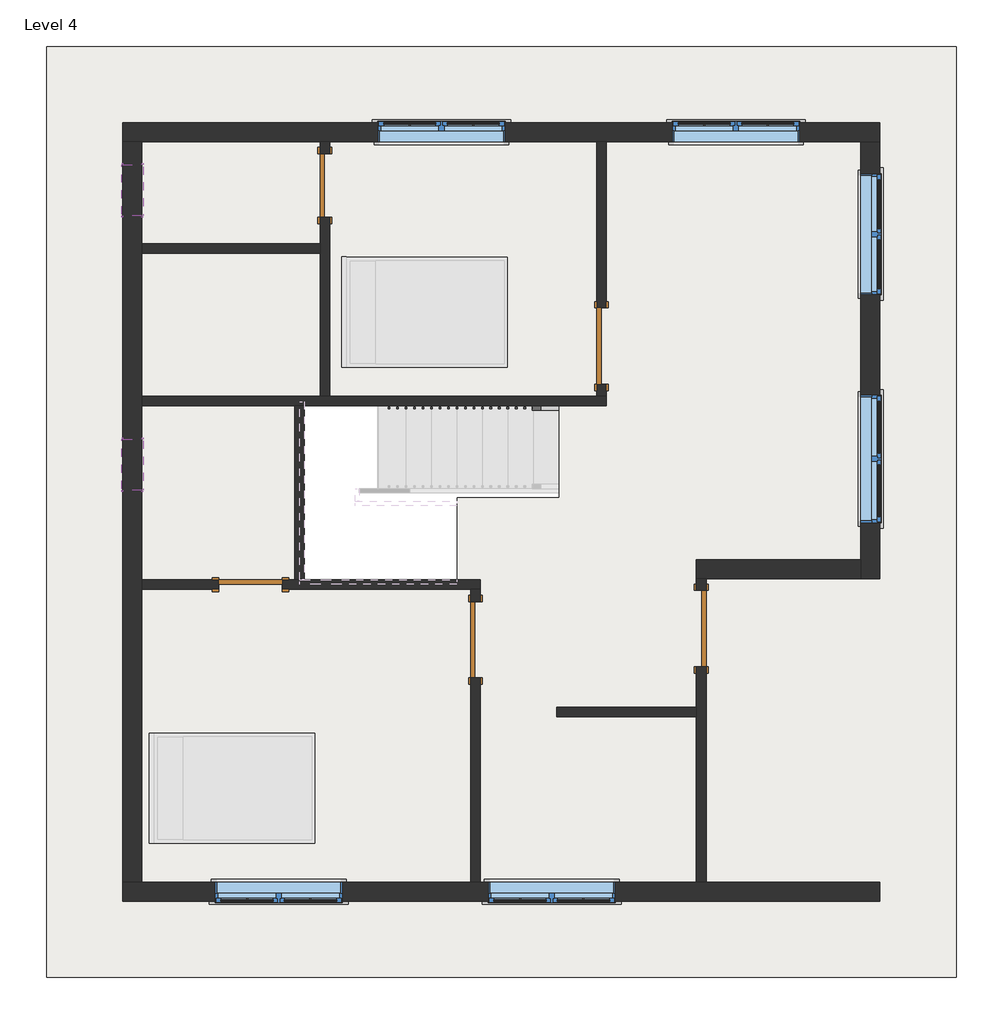
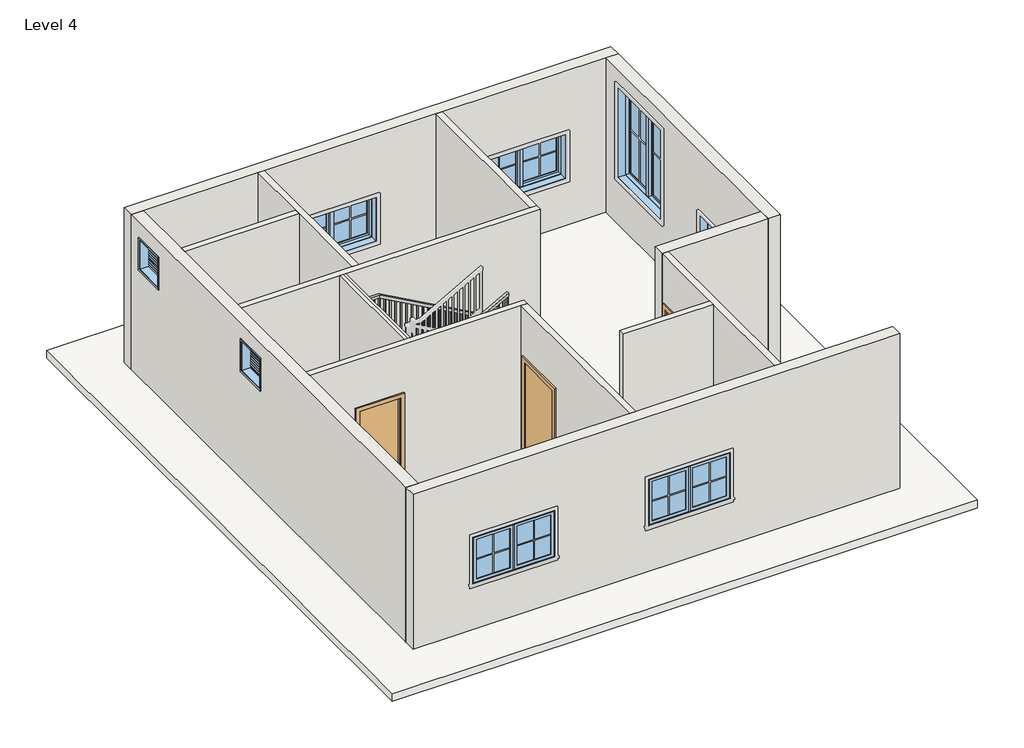
# One storey, part 1 of 2: 14 walls, 8 windows, 5 doors, 1 railing, 1 roof.
"""IFC4 building model written with IfcOpenShell, lengths in millimetres."""

from ifc_helpers import new_model, si_unit, frame, origin, place, context, project, spatial, polyline, outline, extrude, faceted_brep, transform, mapped, element, save
from components import single_flush_3_17d80c48, single_flush_3_5e62189b, door_d8f5dbb5, window_9ac97e1a, window_c1d95f0f, window_f2d8fef0

model = new_model("IFC4")

# Units and contexts
model_context = context("Model", 3, world=origin())
ifc_project = project(units=[si_unit("LENGTHUNIT", "METRE", prefix="MILLI")], contexts=[model_context])

# Site, building, storey
site = spatial("IfcSite", under=ifc_project)
building = spatial("IfcBuilding", under=site)
storey = spatial("IfcBuildingStorey", under=building, Name="Level 4", Elevation=9448.8)

# Doors
placement = place(None, origin())
single_flush_3_shape = single_flush_3_17d80c48(model_context)
element("IfcDoor", 1, ObjectType="Single-Flush : 3'", at=placement, inside=storey, context=model_context, shape_type="MappedRepresentation", body=[
    mapped(single_flush_3_shape, transform((-1566.5130704, -2143.0042021, 9448.8), x_axis=(0.0, 1.0, 0.0), y_axis=(-1.0, 0.0, 0.0), z_axis=(0.0, 0.0, 1.0))),
])
single_flush_3_2_shape = single_flush_3_5e62189b(model_context)
element("IfcDoor", 2, ObjectType="Single-Flush : 3'", at=placement, inside=storey, context=model_context, shape_type="MappedRepresentation", body=[
    mapped(single_flush_3_2_shape, transform((1138.5869296, -2009.6542021, 9448.8), x_axis=(0.0, 1.0, 0.0), y_axis=(-1.0, 0.0, 0.0), z_axis=(0.0, 0.0, 1.0))),
])
element("IfcDoor", 3, ObjectType="Single-Flush : 3'", at=placement, inside=storey, context=model_context, shape_type="MappedRepresentation", body=[
    mapped(single_flush_3_2_shape, transform((-55.2130704, 1374.8957979, 9448.8), x_axis=(0.0, -1.0, 0.0), y_axis=(1.0, 0.0, 0.0), z_axis=(0.0, 0.0, 1.0))),
])
door_shape = door_d8f5dbb5(model_context)
element("IfcDoor", 4, ObjectType="Single-Flush : DOOR 2'6\"", at=placement, inside=storey, context=model_context, shape_type="MappedRepresentation", body=[
    mapped(door_shape, transform((-3369.9130704, 3298.9457979, 9448.8), x_axis=(0.0, 1.0, 0.0), y_axis=(-1.0, 0.0, 0.0), z_axis=(0.0, 0.0, 1.0))),
])
element("IfcDoor", 5, ObjectType="Single-Flush : DOOR 2'6\"", at=placement, inside=storey, context=model_context, shape_type="MappedRepresentation", body=[
    mapped(door_shape, transform((-4258.9130704, -1482.6042021, 9448.8), x_axis=(1.0, 0.0, 0.0), y_axis=(0.0, 1.0, 0.0), z_axis=(0.0, 0.0, 1.0))),
])

# Railing
element("IfcRailing", 6, ObjectType="Handrail - Rectangular", at=placement, inside=storey, context=model_context, shape_type="SolidModel", body=[
    faceted_brep([(-569.5630704, 606.5457979, 10532.5333333), (-569.5630704, 606.5457979, 10474.420221), (-569.5630704, 657.3457979, 10474.420221), (-569.5630704, 657.3457979, 10532.5333333), (-3007.9630704, 606.5457979, 11887.2), (-3021.1266727, 606.5457979, 11836.4), (-3021.1266727, 657.3457979, 11836.4), (-3007.9630704, 657.3457979, 11887.2), (-3566.7630704, 606.5457979, 11887.2), (-3566.7630704, 606.5457979, 11836.4), (-3617.5630704, 657.3457979, 11836.4), (-3617.5630704, 657.3457979, 11887.2), (-3566.7630704, -1374.6542021, 11887.2), (-3566.7630704, -1374.6542021, 11836.4), (-3617.5630704, -1425.4542021, 11836.4), (-3617.5630704, -1425.4542021, 11887.2), (-3312.7630704, -1374.6542021, 11887.2), (-3299.5994682, -1374.6542021, 11836.4), (-3299.5994682, -1425.4542021, 11836.4), (-3312.7630704, -1425.4542021, 11887.2), (-1788.7630704, -1374.6542021, 12733.8666667), (-1788.7630704, -1425.4542021, 12733.8666667), (-1788.7630704, -1425.4542021, 12675.7535543), (-1788.7630704, -1374.6542021, 12675.7535543)], [[[0, 1, 2, 3]], [[1, 0, 4, 5]], [[2, 1, 5, 6]], [[3, 2, 6, 7]], [[0, 3, 7, 4]], [[5, 4, 8, 9]], [[6, 5, 9, 10]], [[7, 6, 10, 11]], [[4, 7, 11, 8]], [[9, 8, 12, 13]], [[10, 9, 13, 14]], [[11, 10, 14, 15]], [[8, 11, 15, 12]], [[13, 12, 16, 17]], [[14, 13, 17, 18]], [[15, 14, 18, 19]], [[12, 15, 19, 16]], [[20, 21, 22, 23]], [[17, 16, 20, 23]], [[18, 17, 23, 22]], [[19, 18, 22, 21]], [[16, 19, 21, 20]]]),
    extrude(outline(polyline([(12638.7118876, -1855.4380704), (12628.1285543, -1874.4880704), (11650.1333333, -1874.4880704), (11650.1333333, -1855.4380704), (12638.7118876, -1855.4380704)])), frame((0.0, -1409.5792021, 0.0), z_axis=(0.0, 1.0, 0.0), x_axis=(0.0, 0.0, 1.0)), (0.0, 0.0, 1.0), 19.05),
    extrude(outline(polyline([(12582.2674432, -1957.0380704), (12571.6841099, -1976.0880704), (11650.1333333, -1976.0880704), (11650.1333333, -1957.0380704), (12582.2674432, -1957.0380704)])), frame((0.0, -1409.5792021, 0.0), z_axis=(0.0, 1.0, 0.0), x_axis=(0.0, 0.0, 1.0)), (0.0, 0.0, 1.0), 19.05),
    extrude(outline(polyline([(12525.8229988, -2058.6380704), (12515.2396654, -2077.6880704), (11650.1333333, -2077.6880704), (11650.1333333, -2058.6380704), (12525.8229988, -2058.6380704)])), frame((0.0, -1409.5792021, 0.0), z_axis=(0.0, 1.0, 0.0), x_axis=(0.0, 0.0, 1.0)), (0.0, 0.0, 1.0), 19.05),
    extrude(outline(polyline([(12469.3785543, -2160.2380704), (12458.795221, -2179.2880704), (11480.8, -2179.2880704), (11480.8, -2160.2380704), (12469.3785543, -2160.2380704)])), frame((0.0, -1409.5792021, 0.0), z_axis=(0.0, 1.0, 0.0), x_axis=(0.0, 0.0, 1.0)), (0.0, 0.0, 1.0), 19.05),
    extrude(outline(polyline([(12412.9341099, -2261.8380704), (12402.3507765, -2280.8880704), (11480.8, -2280.8880704), (11480.8, -2261.8380704), (12412.9341099, -2261.8380704)])), frame((0.0, -1409.5792021, 0.0), z_axis=(0.0, 1.0, 0.0), x_axis=(0.0, 0.0, 1.0)), (0.0, 0.0, 1.0), 19.05),
    extrude(outline(polyline([(12356.4896654, -2363.4380704), (12345.9063321, -2382.4880704), (11480.8, -2382.4880704), (11480.8, -2363.4380704), (12356.4896654, -2363.4380704)])), frame((0.0, -1409.5792021, 0.0), z_axis=(0.0, 1.0, 0.0), x_axis=(0.0, 0.0, 1.0)), (0.0, 0.0, 1.0), 19.05),
    extrude(outline(polyline([(12300.045221, -2465.0380704), (12289.4618876, -2484.0880704), (11311.4666667, -2484.0880704), (11311.4666667, -2465.0380704), (12300.045221, -2465.0380704)])), frame((0.0, -1409.5792021, 0.0), z_axis=(0.0, 1.0, 0.0), x_axis=(0.0, 0.0, 1.0)), (0.0, 0.0, 1.0), 19.05),
    extrude(outline(polyline([(12243.6007765, -2566.6380704), (12233.0174432, -2585.6880704), (11311.4666667, -2585.6880704), (11311.4666667, -2566.6380704), (12243.6007765, -2566.6380704)])), frame((0.0, -1409.5792021, 0.0), z_axis=(0.0, 1.0, 0.0), x_axis=(0.0, 0.0, 1.0)), (0.0, 0.0, 1.0), 19.05),
    extrude(outline(polyline([(12187.1563321, -2668.2380704), (12176.5729988, -2687.2880704), (11311.4666667, -2687.2880704), (11311.4666667, -2668.2380704), (12187.1563321, -2668.2380704)])), frame((0.0, -1409.5792021, 0.0), z_axis=(0.0, 1.0, 0.0), x_axis=(0.0, 0.0, 1.0)), (0.0, 0.0, 1.0), 19.05),
    extrude(outline(polyline([(12130.7118876, -2769.8380704), (12120.1285543, -2788.8880704), (11142.1333333, -2788.8880704), (11142.1333333, -2769.8380704), (12130.7118876, -2769.8380704)])), frame((0.0, -1409.5792021, 0.0), z_axis=(0.0, 1.0, 0.0), x_axis=(0.0, 0.0, 1.0)), (0.0, 0.0, 1.0), 19.05),
    extrude(outline(polyline([(12074.2674432, -2871.4380704), (12063.6841099, -2890.4880704), (11142.1333333, -2890.4880704), (11142.1333333, -2871.4380704), (12074.2674432, -2871.4380704)])), frame((0.0, -1409.5792021, 0.0), z_axis=(0.0, 1.0, 0.0), x_axis=(0.0, 0.0, 1.0)), (0.0, 0.0, 1.0), 19.05),
    extrude(outline(polyline([(12017.8229988, -2973.0380704), (12007.2396654, -2992.0880704), (11142.1333333, -2992.0880704), (11142.1333333, -2973.0380704), (12017.8229988, -2973.0380704)])), frame((0.0, -1409.5792021, 0.0), z_axis=(0.0, 1.0, 0.0), x_axis=(0.0, 0.0, 1.0)), (0.0, 0.0, 1.0), 19.05),
    extrude(outline(polyline([(11961.3785543, -3074.6380704), (11950.795221, -3093.6880704), (10972.8, -3093.6880704), (10972.8, -3074.6380704), (11961.3785543, -3074.6380704)])), frame((0.0, -1409.5792021, 0.0), z_axis=(0.0, 1.0, 0.0), x_axis=(0.0, 0.0, 1.0)), (0.0, 0.0, 1.0), 19.05),
    extrude(outline(polyline([(11904.9341099, -3176.2380704), (11894.3507765, -3195.2880704), (10972.8, -3195.2880704), (10972.8, -3176.2380704), (11904.9341099, -3176.2380704)])), frame((0.0, -1409.5792021, 0.0), z_axis=(0.0, 1.0, 0.0), x_axis=(0.0, 0.0, 1.0)), (0.0, 0.0, 1.0), 19.05),
    extrude(outline(polyline([(11848.4896654, -3277.8380704), (11837.9063321, -3296.8880704), (10972.8, -3296.8880704), (10972.8, -3277.8380704), (11848.4896654, -3277.8380704)])), frame((0.0, -1409.5792021, 0.0), z_axis=(0.0, 1.0, 0.0), x_axis=(0.0, 0.0, 1.0)), (0.0, 0.0, 1.0), 19.05),
    extrude(outline(polyline([(-3398.4880704, -1409.5792021), (-3398.4880704, -1390.5292021), (-3379.4380704, -1390.5292021), (-3379.4380704, -1409.5792021), (-3398.4880704, -1409.5792021)])), frame((0.0, 0.0, 10972.8), z_axis=(0.0, 0.0, 1.0), x_axis=(1.0, 0.0, 0.0)), (0.0, 0.0, 1.0), 863.6),
    extrude(outline(polyline([(-3500.0880704, -1409.5792021), (-3500.0880704, -1390.5292021), (-3481.0380704, -1390.5292021), (-3481.0380704, -1409.5792021), (-3500.0880704, -1409.5792021)])), frame((0.0, 0.0, 10972.8), z_axis=(0.0, 0.0, 1.0), x_axis=(1.0, 0.0, 0.0)), (0.0, 0.0, 1.0), 863.6),
    extrude(outline(polyline([(-3601.6880704, -1288.9292021), (-3582.6380704, -1288.9292021), (-3582.6380704, -1307.9792021), (-3601.6880704, -1307.9792021), (-3601.6880704, -1288.9292021)])), frame((0.0, 0.0, 10972.8), z_axis=(0.0, 0.0, 1.0), x_axis=(1.0, 0.0, 0.0)), (0.0, 0.0, 1.0), 863.6),
    extrude(outline(polyline([(-3601.6880704, -1187.3292021), (-3582.6380704, -1187.3292021), (-3582.6380704, -1206.3792021), (-3601.6880704, -1206.3792021), (-3601.6880704, -1187.3292021)])), frame((0.0, 0.0, 10972.8), z_axis=(0.0, 0.0, 1.0), x_axis=(1.0, 0.0, 0.0)), (0.0, 0.0, 1.0), 863.6),
    extrude(outline(polyline([(-3601.6880704, -1085.7292021), (-3582.6380704, -1085.7292021), (-3582.6380704, -1104.7792021), (-3601.6880704, -1104.7792021), (-3601.6880704, -1085.7292021)])), frame((0.0, 0.0, 10972.8), z_axis=(0.0, 0.0, 1.0), x_axis=(1.0, 0.0, 0.0)), (0.0, 0.0, 1.0), 863.6),
    extrude(outline(polyline([(-3601.6880704, -984.1292021), (-3582.6380704, -984.1292021), (-3582.6380704, -1003.1792021), (-3601.6880704, -1003.1792021), (-3601.6880704, -984.1292021)])), frame((0.0, 0.0, 10972.8), z_axis=(0.0, 0.0, 1.0), x_axis=(1.0, 0.0, 0.0)), (0.0, 0.0, 1.0), 863.6),
    extrude(outline(polyline([(-3601.6880704, -882.5292021), (-3582.6380704, -882.5292021), (-3582.6380704, -901.5792021), (-3601.6880704, -901.5792021), (-3601.6880704, -882.5292021)])), frame((0.0, 0.0, 10972.8), z_axis=(0.0, 0.0, 1.0), x_axis=(1.0, 0.0, 0.0)), (0.0, 0.0, 1.0), 863.6),
    extrude(outline(polyline([(-3601.6880704, -780.9292021), (-3582.6380704, -780.9292021), (-3582.6380704, -799.9792021), (-3601.6880704, -799.9792021), (-3601.6880704, -780.9292021)])), frame((0.0, 0.0, 10972.8), z_axis=(0.0, 0.0, 1.0), x_axis=(1.0, 0.0, 0.0)), (0.0, 0.0, 1.0), 863.6),
    extrude(outline(polyline([(-3601.6880704, -679.3292021), (-3582.6380704, -679.3292021), (-3582.6380704, -698.3792021), (-3601.6880704, -698.3792021), (-3601.6880704, -679.3292021)])), frame((0.0, 0.0, 10972.8), z_axis=(0.0, 0.0, 1.0), x_axis=(1.0, 0.0, 0.0)), (0.0, 0.0, 1.0), 863.6),
    extrude(outline(polyline([(-3601.6880704, -577.7292021), (-3582.6380704, -577.7292021), (-3582.6380704, -596.7792021), (-3601.6880704, -596.7792021), (-3601.6880704, -577.7292021)])), frame((0.0, 0.0, 10972.8), z_axis=(0.0, 0.0, 1.0), x_axis=(1.0, 0.0, 0.0)), (0.0, 0.0, 1.0), 863.6),
    extrude(outline(polyline([(-3601.6880704, -476.1292021), (-3582.6380704, -476.1292021), (-3582.6380704, -495.1792021), (-3601.6880704, -495.1792021), (-3601.6880704, -476.1292021)])), frame((0.0, 0.0, 10972.8), z_axis=(0.0, 0.0, 1.0), x_axis=(1.0, 0.0, 0.0)), (0.0, 0.0, 1.0), 863.6),
    extrude(outline(polyline([(-3601.6880704, -374.5292021), (-3582.6380704, -374.5292021), (-3582.6380704, -393.5792021), (-3601.6880704, -393.5792021), (-3601.6880704, -374.5292021)])), frame((0.0, 0.0, 10972.8), z_axis=(0.0, 0.0, 1.0), x_axis=(1.0, 0.0, 0.0)), (0.0, 0.0, 1.0), 863.6),
    extrude(outline(polyline([(-3601.6880704, -272.9292021), (-3582.6380704, -272.9292021), (-3582.6380704, -291.9792021), (-3601.6880704, -291.9792021), (-3601.6880704, -272.9292021)])), frame((0.0, 0.0, 10972.8), z_axis=(0.0, 0.0, 1.0), x_axis=(1.0, 0.0, 0.0)), (0.0, 0.0, 1.0), 863.6),
    extrude(outline(polyline([(-3601.6880704, -171.3292021), (-3582.6380704, -171.3292021), (-3582.6380704, -190.3792021), (-3601.6880704, -190.3792021), (-3601.6880704, -171.3292021)])), frame((0.0, 0.0, 10972.8), z_axis=(0.0, 0.0, 1.0), x_axis=(1.0, 0.0, 0.0)), (0.0, 0.0, 1.0), 863.6),
    extrude(outline(polyline([(-3601.6880704, -69.7292021), (-3582.6380704, -69.7292021), (-3582.6380704, -88.7792021), (-3601.6880704, -88.7792021), (-3601.6880704, -69.7292021)])), frame((0.0, 0.0, 10972.8), z_axis=(0.0, 0.0, 1.0), x_axis=(1.0, 0.0, 0.0)), (0.0, 0.0, 1.0), 863.6),
    extrude(outline(polyline([(-3601.6880704, 31.8707979), (-3582.6380704, 31.8707979), (-3582.6380704, 12.8207979), (-3601.6880704, 12.8207979), (-3601.6880704, 31.8707979)])), frame((0.0, 0.0, 10972.8), z_axis=(0.0, 0.0, 1.0), x_axis=(1.0, 0.0, 0.0)), (0.0, 0.0, 1.0), 863.6),
    extrude(outline(polyline([(-3601.6880704, 133.4707979), (-3582.6380704, 133.4707979), (-3582.6380704, 114.4207979), (-3601.6880704, 114.4207979), (-3601.6880704, 133.4707979)])), frame((0.0, 0.0, 10972.8), z_axis=(0.0, 0.0, 1.0), x_axis=(1.0, 0.0, 0.0)), (0.0, 0.0, 1.0), 863.6),
    extrude(outline(polyline([(-3601.6880704, 235.0707979), (-3582.6380704, 235.0707979), (-3582.6380704, 216.0207979), (-3601.6880704, 216.0207979), (-3601.6880704, 235.0707979)])), frame((0.0, 0.0, 10972.8), z_axis=(0.0, 0.0, 1.0), x_axis=(1.0, 0.0, 0.0)), (0.0, 0.0, 1.0), 863.6),
    extrude(outline(polyline([(-3601.6880704, 336.6707979), (-3582.6380704, 336.6707979), (-3582.6380704, 317.6207979), (-3601.6880704, 317.6207979), (-3601.6880704, 336.6707979)])), frame((0.0, 0.0, 10972.8), z_axis=(0.0, 0.0, 1.0), x_axis=(1.0, 0.0, 0.0)), (0.0, 0.0, 1.0), 863.6),
    extrude(outline(polyline([(-3601.6880704, 438.2707979), (-3582.6380704, 438.2707979), (-3582.6380704, 419.2207979), (-3601.6880704, 419.2207979), (-3601.6880704, 438.2707979)])), frame((0.0, 0.0, 10972.8), z_axis=(0.0, 0.0, 1.0), x_axis=(1.0, 0.0, 0.0)), (0.0, 0.0, 1.0), 863.6),
    extrude(outline(polyline([(-3601.6880704, 539.8707979), (-3582.6380704, 539.8707979), (-3582.6380704, 520.8207979), (-3601.6880704, 520.8207979), (-3601.6880704, 539.8707979)])), frame((0.0, 0.0, 10972.8), z_axis=(0.0, 0.0, 1.0), x_axis=(1.0, 0.0, 0.0)), (0.0, 0.0, 1.0), 863.6),
    extrude(outline(polyline([(-3506.4380704, 641.4707979), (-3506.4380704, 622.4207979), (-3525.4880704, 622.4207979), (-3525.4880704, 641.4707979), (-3506.4380704, 641.4707979)])), frame((0.0, 0.0, 10972.8), z_axis=(0.0, 0.0, 1.0), x_axis=(1.0, 0.0, 0.0)), (0.0, 0.0, 1.0), 863.6),
    extrude(outline(polyline([(-3404.8380704, 641.4707979), (-3404.8380704, 622.4207979), (-3423.8880704, 622.4207979), (-3423.8880704, 641.4707979), (-3404.8380704, 641.4707979)])), frame((0.0, 0.0, 10972.8), z_axis=(0.0, 0.0, 1.0), x_axis=(1.0, 0.0, 0.0)), (0.0, 0.0, 1.0), 863.6),
    extrude(outline(polyline([(-3303.2380704, 641.4707979), (-3303.2380704, 622.4207979), (-3322.2880704, 622.4207979), (-3322.2880704, 641.4707979), (-3303.2380704, 641.4707979)])), frame((0.0, 0.0, 10972.8), z_axis=(0.0, 0.0, 1.0), x_axis=(1.0, 0.0, 0.0)), (0.0, 0.0, 1.0), 863.6),
    extrude(outline(polyline([(-3201.6380704, 641.4707979), (-3201.6380704, 622.4207979), (-3220.6880704, 622.4207979), (-3220.6880704, 641.4707979), (-3201.6380704, 641.4707979)])), frame((0.0, 0.0, 10972.8), z_axis=(0.0, 0.0, 1.0), x_axis=(1.0, 0.0, 0.0)), (0.0, 0.0, 1.0), 863.6),
    extrude(outline(polyline([(-3100.0380704, 641.4707979), (-3100.0380704, 622.4207979), (-3119.0880704, 622.4207979), (-3119.0880704, 641.4707979), (-3100.0380704, 641.4707979)])), frame((0.0, 0.0, 10972.8), z_axis=(0.0, 0.0, 1.0), x_axis=(1.0, 0.0, 0.0)), (0.0, 0.0, 1.0), 863.6),
    extrude(outline(polyline([(11823.795221, -2998.4380704), (11834.3785543, -3017.4880704), (10972.8, -3017.4880704), (10972.8, -2998.4380704), (11823.795221, -2998.4380704)])), frame((0.0, 622.4207979, 0.0), z_axis=(0.0, 1.0, 0.0), x_axis=(0.0, 0.0, 1.0)), (0.0, 0.0, 1.0), 19.05),
    extrude(outline(polyline([(11767.3507765, -2896.8380704), (11777.9341099, -2915.8880704), (10803.4666667, -2915.8880704), (10803.4666667, -2896.8380704), (11767.3507765, -2896.8380704)])), frame((0.0, 622.4207979, 0.0), z_axis=(0.0, 1.0, 0.0), x_axis=(0.0, 0.0, 1.0)), (0.0, 0.0, 1.0), 19.05),
    extrude(outline(polyline([(11710.9063321, -2795.2380704), (11721.4896654, -2814.2880704), (10803.4666667, -2814.2880704), (10803.4666667, -2795.2380704), (11710.9063321, -2795.2380704)])), frame((0.0, 622.4207979, 0.0), z_axis=(0.0, 1.0, 0.0), x_axis=(0.0, 0.0, 1.0)), (0.0, 0.0, 1.0), 19.05),
    extrude(outline(polyline([(11654.4618876, -2693.6380704), (11665.045221, -2712.6880704), (10803.4666667, -2712.6880704), (10803.4666667, -2693.6380704), (11654.4618876, -2693.6380704)])), frame((0.0, 622.4207979, 0.0), z_axis=(0.0, 1.0, 0.0), x_axis=(0.0, 0.0, 1.0)), (0.0, 0.0, 1.0), 19.05),
    extrude(outline(polyline([(11598.0174432, -2592.0380704), (11608.6007765, -2611.0880704), (10634.1333333, -2611.0880704), (10634.1333333, -2592.0380704), (11598.0174432, -2592.0380704)])), frame((0.0, 622.4207979, 0.0), z_axis=(0.0, 1.0, 0.0), x_axis=(0.0, 0.0, 1.0)), (0.0, 0.0, 1.0), 19.05),
    extrude(outline(polyline([(11541.5729988, -2490.4380704), (11552.1563321, -2509.4880704), (10634.1333333, -2509.4880704), (10634.1333333, -2490.4380704), (11541.5729988, -2490.4380704)])), frame((0.0, 622.4207979, 0.0), z_axis=(0.0, 1.0, 0.0), x_axis=(0.0, 0.0, 1.0)), (0.0, 0.0, 1.0), 19.05),
    extrude(outline(polyline([(11485.1285543, -2388.8380704), (11495.7118876, -2407.8880704), (10634.1333333, -2407.8880704), (10634.1333333, -2388.8380704), (11485.1285543, -2388.8380704)])), frame((0.0, 622.4207979, 0.0), z_axis=(0.0, 1.0, 0.0), x_axis=(0.0, 0.0, 1.0)), (0.0, 0.0, 1.0), 19.05),
    extrude(outline(polyline([(11428.6841099, -2287.2380704), (11439.2674432, -2306.2880704), (10464.8, -2306.2880704), (10464.8, -2287.2380704), (11428.6841099, -2287.2380704)])), frame((0.0, 622.4207979, 0.0), z_axis=(0.0, 1.0, 0.0), x_axis=(0.0, 0.0, 1.0)), (0.0, 0.0, 1.0), 19.05),
    extrude(outline(polyline([(11372.2396654, -2185.6380704), (11382.8229988, -2204.6880704), (10464.8, -2204.6880704), (10464.8, -2185.6380704), (11372.2396654, -2185.6380704)])), frame((0.0, 622.4207979, 0.0), z_axis=(0.0, 1.0, 0.0), x_axis=(0.0, 0.0, 1.0)), (0.0, 0.0, 1.0), 19.05),
    extrude(outline(polyline([(11315.795221, -2084.0380704), (11326.3785543, -2103.0880704), (10464.8, -2103.0880704), (10464.8, -2084.0380704), (11315.795221, -2084.0380704)])), frame((0.0, 622.4207979, 0.0), z_axis=(0.0, 1.0, 0.0), x_axis=(0.0, 0.0, 1.0)), (0.0, 0.0, 1.0), 19.05),
    extrude(outline(polyline([(11259.3507765, -1982.4380704), (11269.9341099, -2001.4880704), (10295.4666667, -2001.4880704), (10295.4666667, -1982.4380704), (11259.3507765, -1982.4380704)])), frame((0.0, 622.4207979, 0.0), z_axis=(0.0, 1.0, 0.0), x_axis=(0.0, 0.0, 1.0)), (0.0, 0.0, 1.0), 19.05),
    extrude(outline(polyline([(11202.9063321, -1880.8380704), (11213.4896654, -1899.8880704), (10295.4666667, -1899.8880704), (10295.4666667, -1880.8380704), (11202.9063321, -1880.8380704)])), frame((0.0, 622.4207979, 0.0), z_axis=(0.0, 1.0, 0.0), x_axis=(0.0, 0.0, 1.0)), (0.0, 0.0, 1.0), 19.05),
    extrude(outline(polyline([(11146.4618876, -1779.2380704), (11157.045221, -1798.2880704), (10295.4666667, -1798.2880704), (10295.4666667, -1779.2380704), (11146.4618876, -1779.2380704)])), frame((0.0, 622.4207979, 0.0), z_axis=(0.0, 1.0, 0.0), x_axis=(0.0, 0.0, 1.0)), (0.0, 0.0, 1.0), 19.05),
    extrude(outline(polyline([(11090.0174432, -1677.6380704), (11100.6007765, -1696.6880704), (10126.1333333, -1696.6880704), (10126.1333333, -1677.6380704), (11090.0174432, -1677.6380704)])), frame((0.0, 622.4207979, 0.0), z_axis=(0.0, 1.0, 0.0), x_axis=(0.0, 0.0, 1.0)), (0.0, 0.0, 1.0), 19.05),
    extrude(outline(polyline([(11033.5729988, -1576.0380704), (11044.1563321, -1595.0880704), (10126.1333333, -1595.0880704), (10126.1333333, -1576.0380704), (11033.5729988, -1576.0380704)])), frame((0.0, 622.4207979, 0.0), z_axis=(0.0, 1.0, 0.0), x_axis=(0.0, 0.0, 1.0)), (0.0, 0.0, 1.0), 19.05),
    extrude(outline(polyline([(10977.1285543, -1474.4380704), (10987.7118876, -1493.4880704), (10126.1333333, -1493.4880704), (10126.1333333, -1474.4380704), (10977.1285543, -1474.4380704)])), frame((0.0, 622.4207979, 0.0), z_axis=(0.0, 1.0, 0.0), x_axis=(0.0, 0.0, 1.0)), (0.0, 0.0, 1.0), 19.05),
    extrude(outline(polyline([(10920.6841099, -1372.8380704), (10931.2674432, -1391.8880704), (9956.8, -1391.8880704), (9956.8, -1372.8380704), (10920.6841099, -1372.8380704)])), frame((0.0, 622.4207979, 0.0), z_axis=(0.0, 1.0, 0.0), x_axis=(0.0, 0.0, 1.0)), (0.0, 0.0, 1.0), 19.05),
    extrude(outline(polyline([(10864.2396654, -1271.2380704), (10874.8229988, -1290.2880704), (9956.8, -1290.2880704), (9956.8, -1271.2380704), (10864.2396654, -1271.2380704)])), frame((0.0, 622.4207979, 0.0), z_axis=(0.0, 1.0, 0.0), x_axis=(0.0, 0.0, 1.0)), (0.0, 0.0, 1.0), 19.05),
    extrude(outline(polyline([(10807.795221, -1169.6380704), (10818.3785543, -1188.6880704), (9956.8, -1188.6880704), (9956.8, -1169.6380704), (10807.795221, -1169.6380704)])), frame((0.0, 622.4207979, 0.0), z_axis=(0.0, 1.0, 0.0), x_axis=(0.0, 0.0, 1.0)), (0.0, 0.0, 1.0), 19.05),
    extrude(outline(polyline([(10751.3507765, -1068.0380704), (10761.9341099, -1087.0880704), (9787.4666667, -1087.0880704), (9787.4666667, -1068.0380704), (10751.3507765, -1068.0380704)])), frame((0.0, 622.4207979, 0.0), z_axis=(0.0, 1.0, 0.0), x_axis=(0.0, 0.0, 1.0)), (0.0, 0.0, 1.0), 19.05),
    extrude(outline(polyline([(10694.9063321, -966.4380704), (10705.4896654, -985.4880704), (9787.4666667, -985.4880704), (9787.4666667, -966.4380704), (10694.9063321, -966.4380704)])), frame((0.0, 622.4207979, 0.0), z_axis=(0.0, 1.0, 0.0), x_axis=(0.0, 0.0, 1.0)), (0.0, 0.0, 1.0), 19.05),
    extrude(outline(polyline([(10638.4618876, -864.8380704), (10649.045221, -883.8880704), (9787.4666667, -883.8880704), (9787.4666667, -864.8380704), (10638.4618876, -864.8380704)])), frame((0.0, 622.4207979, 0.0), z_axis=(0.0, 1.0, 0.0), x_axis=(0.0, 0.0, 1.0)), (0.0, 0.0, 1.0), 19.05),
    extrude(outline(polyline([(10582.0174432, -763.2380704), (10592.6007765, -782.2880704), (9618.1333333, -782.2880704), (9618.1333333, -763.2380704), (10582.0174432, -763.2380704)])), frame((0.0, 622.4207979, 0.0), z_axis=(0.0, 1.0, 0.0), x_axis=(0.0, 0.0, 1.0)), (0.0, 0.0, 1.0), 19.05),
    extrude(outline(polyline([(10525.5729988, -661.6380704), (10536.1563321, -680.6880704), (9618.1333333, -680.6880704), (9618.1333333, -661.6380704), (10525.5729988, -661.6380704)])), frame((0.0, 622.4207979, 0.0), z_axis=(0.0, 1.0, 0.0), x_axis=(0.0, 0.0, 1.0)), (0.0, 0.0, 1.0), 19.05),
    extrude(outline(polyline([(-3601.6880704, -1390.5292021), (-3582.6380704, -1390.5292021), (-3582.6380704, -1409.5792021), (-3601.6880704, -1409.5792021), (-3601.6880704, -1390.5292021)])), frame((0.0, 0.0, 10972.8), z_axis=(0.0, 0.0, 1.0), x_axis=(1.0, 0.0, 0.0)), (0.0, 0.0, 1.0), 863.6),
    extrude(outline(polyline([(-3582.6380704, 641.4707979), (-3582.6380704, 622.4207979), (-3601.6880704, 622.4207979), (-3601.6880704, 641.4707979), (-3582.6380704, 641.4707979)])), frame((0.0, 0.0, 10972.8), z_axis=(0.0, 0.0, 1.0), x_axis=(1.0, 0.0, 0.0)), (0.0, 0.0, 1.0), 863.6),
    extrude(outline(polyline([(12675.7535543, -1788.7630704), (12665.170221, -1807.8130704), (11650.1333333, -1807.8130704), (11650.1333333, -1788.7630704), (12675.7535543, -1788.7630704)])), frame((0.0, -1409.5792021, 0.0), z_axis=(0.0, 1.0, 0.0), x_axis=(0.0, 0.0, 1.0)), (0.0, 0.0, 1.0), 19.05),
    extrude(outline(polyline([(10474.420221, -569.5630704), (10485.0035543, -588.6130704), (9618.1333333, -588.6130704), (9618.1333333, -569.5630704), (10474.420221, -569.5630704)])), frame((0.0, 622.4207979, 0.0), z_axis=(0.0, 1.0, 0.0), x_axis=(0.0, 0.0, 1.0)), (0.0, 0.0, 1.0), 19.05),
])

# Roof
element("IfcRoof", 7, ObjectType="roof 6\"", at=placement, inside=storey, context=model_context, shape_type="SweptSolid", body=[
    extrude(outline(polyline([(4192.9369296, 4962.6457979), (4192.9369296, -6187.9542021), (-6703.6630704, -6187.9542021), (-6703.6630704, 4962.6457979), (4192.9369296, 4962.6457979)]), holes=[polyline([(-3668.3630704, 708.1457979), (-3668.3630704, -1476.2542021), (-1788.7630704, -1476.2542021), (-1788.7630704, -434.8542021), (-569.5630704, -434.8542021), (-569.5630704, 708.1457979), (-3668.3630704, 708.1457979)])]), frame((0.0, 0.0, 9296.4), z_axis=(0.0, 0.0, 1.0), x_axis=(1.0, 0.0, 0.0)), (0.0, 0.0, 1.0), 152.4),
])

# Walls
element("IfcWall", 8, ObjectType="WALL 4.5\"", at=placement, inside=storey, context=model_context, shape_type="Brep", body=[
    faceted_brep([(-3427.0630704, 3819.6457979, 9448.8), (-3427.0630704, 3679.9457979, 9448.8), (-3427.0630704, 3679.9457979, 11480.8), (-3427.0630704, 2917.9457979, 11480.8), (-3427.0630704, 2917.9457979, 9448.8), (-3427.0630704, 2600.4457979, 9448.8), (-3427.0630704, 2486.1457979, 9448.8), (-3427.0630704, 771.6457979, 9448.8), (-3427.0630704, 771.6457979, 12496.8), (-3427.0630704, 2486.1457979, 12496.8), (-3427.0630704, 2600.4457979, 12496.8), (-3427.0630704, 3819.6457979, 12496.8), (-3312.7630704, 3679.9457979, 11480.8), (-3312.7630704, 3679.9457979, 9448.8), (-3312.7630704, 3819.6457979, 9448.8), (-3312.7630704, 3819.6457979, 12496.8), (-3312.7630704, 771.6457979, 12496.8), (-3312.7630704, 771.6457979, 9448.8), (-3312.7630704, 2917.9457979, 9448.8), (-3312.7630704, 2917.9457979, 11480.8)], [[[0, 1, 2, 3, 4, 5, 6, 7, 8, 9, 10, 11]], [[12, 13, 14, 15, 16, 17, 18, 19]], [[18, 17, 7, 6, 5, 4]], [[14, 13, 1, 0]], [[0, 11, 15, 14]], [[8, 7, 17, 16]], [[2, 1, 13, 12]], [[3, 2, 12, 19]], [[4, 3, 19, 18]], [[11, 10, 9, 8, 16, 15]]]),
])
element("IfcWall", 9, ObjectType="WALL 4.5\"", at=placement, inside=storey, context=model_context, shape_type="Brep", body=[
    faceted_brep([(-5560.6630704, 657.3457979, 9448.8), (-3731.8630704, 657.3457979, 9448.8), (-3617.5630704, 657.3457979, 9448.8), (1.9369296, 657.3457979, 9448.8), (1.9369296, 657.3457979, 12496.8), (-3617.5630704, 657.3457979, 12496.8), (-3731.8630704, 657.3457979, 12496.8), (-5560.6630704, 657.3457979, 12496.8), (-5560.6630704, 771.6457979, 9448.8), (-5560.6630704, 771.6457979, 12496.8), (-3427.0630704, 771.6457979, 12496.8), (-3312.7630704, 771.6457979, 12496.8), (-112.3630704, 771.6457979, 12496.8), (1.9369296, 771.6457979, 12496.8), (1.9369296, 771.6457979, 9448.8), (-112.3630704, 771.6457979, 9448.8), (-3312.7630704, 771.6457979, 9448.8), (-3427.0630704, 771.6457979, 9448.8)], [[[0, 1, 2, 3, 4, 5, 6, 7]], [[8, 9, 10, 11, 12, 13, 14, 15, 16, 17]], [[3, 2, 1, 0, 8, 17, 16, 15, 14]], [[7, 6, 5, 4, 13, 12, 11, 10, 9]], [[0, 7, 9, 8]], [[4, 3, 14, 13]]]),
])
element("IfcWall", 10, ObjectType="WALL 4.5\"", at=placement, inside=storey, context=model_context, shape_type="SweptSolid", body=[
    extrude(outline(polyline([(917.6957979, 11480.8), (917.6957979, 9448.8), (771.6457979, 9448.8), (771.6457979, 12496.8), (3819.6457979, 12496.8), (3819.6457979, 9448.8), (1832.0957979, 9448.8), (1832.0957979, 11480.8), (917.6957979, 11480.8)])), frame((-112.3630704, 0.0, 0.0), z_axis=(1.0, 0.0, 0.0), x_axis=(0.0, 1.0, 0.0)), (0.0, 0.0, 1.0), 114.3),
])
element("IfcWall", 11, ObjectType="WALL 4.5\"", at=placement, inside=storey, context=model_context, shape_type="SweptSolid", body=[
    extrude(outline(polyline([(-3427.0630704, 2486.1457979), (-5560.6630704, 2486.1457979), (-5560.6630704, 2600.4457979), (-3427.0630704, 2600.4457979), (-3427.0630704, 2486.1457979)])), frame((0.0, 0.0, 9448.8), z_axis=(0.0, 0.0, 1.0), x_axis=(1.0, 0.0, 0.0)), (0.0, 0.0, 1.0), 3048.0),
])
element("IfcWall", 12, ObjectType="WALL 4.5\"", at=placement, inside=storey, context=model_context, shape_type="Brep", body=[
    faceted_brep([(-3877.9130704, -1539.7542021, 11480.8), (-3877.9130704, -1539.7542021, 9448.8), (-1623.6630704, -1539.7542021, 9448.8), (-1509.3630704, -1539.7542021, 9448.8), (-1509.3630704, -1539.7542021, 12496.8), (-1623.6630704, -1539.7542021, 12496.8), (-5560.6630704, -1539.7542021, 12496.8), (-5560.6630704, -1539.7542021, 9448.8), (-4639.9130704, -1539.7542021, 9448.8), (-4639.9130704, -1539.7542021, 11480.8), (-1509.3630704, -1425.4542021, 9448.8), (-3617.5630704, -1425.4542021, 9448.8), (-3731.8630704, -1425.4542021, 9448.8), (-3877.9130704, -1425.4542021, 9448.8), (-3877.9130704, -1425.4542021, 11480.8), (-4639.9130704, -1425.4542021, 11480.8), (-4639.9130704, -1425.4542021, 9448.8), (-5560.6630704, -1425.4542021, 9448.8), (-5560.6630704, -1425.4542021, 12496.8), (-3731.8630704, -1425.4542021, 12496.8), (-3617.5630704, -1425.4542021, 12496.8), (-1509.3630704, -1425.4542021, 12496.8)], [[[0, 1, 2, 3, 4, 5, 6, 7, 8, 9]], [[10, 11, 12, 13, 14, 15, 16, 17, 18, 19, 20, 21]], [[8, 7, 17, 16]], [[3, 2, 1, 13, 12, 11, 10]], [[6, 5, 4, 21, 20, 19, 18]], [[7, 6, 18, 17]], [[4, 3, 10, 21]], [[14, 13, 1, 0]], [[15, 14, 0, 9]], [[16, 15, 9, 8]]]),
])
element("IfcWall", 13, ObjectType="WALL 4.5\"", at=placement, inside=storey, context=model_context, shape_type="SweptSolid", body=[
    extrude(outline(polyline([(-1539.7542021, 9448.8), (-1685.8042021, 9448.8), (-1685.8042021, 11480.8), (-2600.2042021, 11480.8), (-2600.2042021, 9448.8), (-5044.9542021, 9448.8), (-5044.9542021, 12496.8), (-1539.7542021, 12496.8), (-1539.7542021, 9448.8)])), frame((-1623.6630704, 0.0, 0.0), z_axis=(1.0, 0.0, 0.0), x_axis=(0.0, 1.0, 0.0)), (0.0, 0.0, 1.0), 114.3),
])
element("IfcWall", 14, ObjectType="WALL 4.5\"", at=placement, inside=storey, context=model_context, shape_type="Brep", body=[
    faceted_brep([(1195.7369296, -1552.4542021, 11480.8), (1195.7369296, -1552.4542021, 9448.8), (1195.7369296, -1412.7542021, 9448.8), (1195.7369296, -1412.7542021, 12496.8), (1195.7369296, -5044.9542021, 12496.8), (1195.7369296, -5044.9542021, 9448.8), (1195.7369296, -2466.8542021, 9448.8), (1195.7369296, -2466.8542021, 11480.8), (1081.4369296, -1412.7542021, 9448.8), (1081.4369296, -1552.4542021, 9448.8), (1081.4369296, -1552.4542021, 11480.8), (1081.4369296, -2466.8542021, 11480.8), (1081.4369296, -2466.8542021, 9448.8), (1081.4369296, -2948.9967683, 9448.8), (1081.4369296, -3063.2967683, 9448.8), (1081.4369296, -5044.9542021, 9448.8), (1081.4369296, -5044.9542021, 12496.8), (1081.4369296, -3063.2967683, 12496.8), (1081.4369296, -2948.9967683, 12496.8), (1081.4369296, -1412.7542021, 12496.8)], [[[0, 1, 2, 3, 4, 5, 6, 7]], [[8, 9, 10, 11, 12, 13, 14, 15, 16, 17, 18, 19]], [[6, 5, 15, 14, 13, 12]], [[2, 1, 9, 8]], [[3, 2, 8, 19]], [[5, 4, 16, 15]], [[10, 9, 1, 0]], [[11, 10, 0, 7]], [[12, 11, 7, 6]], [[4, 3, 19, 18, 17, 16]]]),
])
element("IfcWall", 15, ObjectType="WALL 4.5\"", at=placement, inside=storey, context=model_context, shape_type="SweptSolid", body=[
    extrude(outline(polyline([(-594.9630704, -2948.9967683), (1081.4369296, -2948.9967683), (1081.4369296, -3063.2967683), (-594.9630704, -3063.2967683), (-594.9630704, -2948.9967683)])), frame((0.0, 0.0, 9448.8), z_axis=(0.0, 0.0, 1.0), x_axis=(1.0, 0.0, 0.0)), (0.0, 0.0, 1.0), 3048.0),
])
element("IfcWall", 16, ObjectType="WALL 4.5\"", at=placement, inside=storey, context=model_context, shape_type="SweptSolid", body=[
    extrude(outline(polyline([(12496.8, -3731.8630704), (9448.8, -3731.8630704), (9448.8, -3617.5630704), (12496.8, -3617.5630704), (12496.8, -3668.3630704), (12496.8, -3731.8630704)])), frame((0.0, -1425.4542021, 0.0), z_axis=(0.0, 1.0, 0.0), x_axis=(0.0, 0.0, 1.0)), (0.0, 0.0, 1.0), 2082.8),
])
element("IfcWall", 17, ObjectType="WALL 9\"", at=placement, inside=storey, context=model_context, shape_type="Brep", body=[
    faceted_brep([(-5789.2630704, 3819.6457979, 9448.8), (-5560.6630704, 3819.6457979, 9448.8), (-3427.0630704, 3819.6457979, 9448.8), (-3312.7630704, 3819.6457979, 9448.8), (-112.3630704, 3819.6457979, 9448.8), (1.9369296, 3819.6457979, 9448.8), (3049.9369296, 3819.6457979, 9448.8), (3278.5369296, 3819.6457979, 9448.8), (3278.5369296, 3819.6457979, 12496.8), (3049.9369296, 3819.6457979, 12496.8), (1.9369296, 3819.6457979, 12496.8), (-112.3630704, 3819.6457979, 12496.8), (-3312.7630704, 3819.6457979, 12496.8), (-3427.0630704, 3819.6457979, 12496.8), (-5560.6630704, 3819.6457979, 12496.8), (-5789.2630704, 3819.6457979, 12496.8), (2316.5119296, 3819.6457979, 11277.6), (2316.5119296, 3819.6457979, 10363.2), (792.5119296, 3819.6457979, 10363.2), (792.5119296, 3819.6457979, 11277.6), (-1210.9130704, 3819.6457979, 11277.6), (-1210.9130704, 3819.6457979, 10363.2), (-2734.9130704, 3819.6457979, 10363.2), (-2734.9130704, 3819.6457979, 11277.6), (-5789.2630704, 4048.2457979, 9448.8), (-5789.2630704, 4048.2457979, 12496.8), (3278.5369296, 4048.2457979, 12496.8), (3278.5369296, 4048.2457979, 9448.8), (2316.5119296, 4048.2457979, 11277.6), (792.5119296, 4048.2457979, 11277.6), (792.5119296, 4048.2457979, 10363.2), (2316.5119296, 4048.2457979, 10363.2), (-1210.9130704, 4048.2457979, 11277.6), (-2734.9130704, 4048.2457979, 11277.6), (-2734.9130704, 4048.2457979, 10363.2), (-1210.9130704, 4048.2457979, 10363.2)], [[[0, 1, 2, 3, 4, 5, 6, 7, 8, 9, 10, 11, 12, 13, 14, 15], [16, 17, 18, 19], [20, 21, 22, 23]], [[24, 25, 26, 27], [28, 29, 30, 31], [32, 33, 34, 35]], [[7, 6, 5, 4, 3, 2, 1, 0, 24, 27]], [[8, 7, 27, 26]], [[0, 15, 25, 24]], [[17, 16, 28, 31]], [[18, 17, 31, 30]], [[19, 18, 30, 29]], [[16, 19, 29, 28]], [[21, 20, 32, 35]], [[22, 21, 35, 34]], [[23, 22, 34, 33]], [[20, 23, 33, 32]], [[15, 14, 13, 12, 11, 10, 9, 8, 26, 25]]]),
])
element("IfcWall", 18, ObjectType="WALL 9\"", at=placement, inside=storey, context=model_context, shape_type="Brep", body=[
    faceted_brep([(3049.9369296, 3819.6457979, 9448.8), (3049.9369296, -1184.1542021, 9448.8), (3049.9369296, -1412.7542021, 9448.8), (3049.9369296, -1412.7542021, 12496.8), (3049.9369296, -1184.1542021, 12496.8), (3049.9369296, 3819.6457979, 12496.8), (3049.9369296, -739.6542021, 11277.6), (3049.9369296, -739.6542021, 10363.2), (3049.9369296, 784.3457979, 10363.2), (3049.9369296, 784.3457979, 11277.6), (3049.9369296, 1990.8457979, 12192.0), (3049.9369296, 1990.8457979, 10363.2), (3049.9369296, 3438.6457979, 10363.2), (3049.9369296, 3438.6457979, 12192.0), (3278.5369296, 3819.6457979, 9448.8), (3278.5369296, 3819.6457979, 12496.8), (3278.5369296, -1412.7542021, 12496.8), (3278.5369296, -1412.7542021, 9448.8), (3278.5369296, -739.6542021, 11277.6), (3278.5369296, 784.3457979, 11277.6), (3278.5369296, 784.3457979, 10363.2), (3278.5369296, -739.6542021, 10363.2), (3278.5369296, 1990.8457979, 12192.0), (3278.5369296, 3438.6457979, 12192.0), (3278.5369296, 3438.6457979, 10363.2), (3278.5369296, 1990.8457979, 10363.2)], [[[0, 1, 2, 3, 4, 5], [6, 7, 8, 9], [10, 11, 12, 13]], [[14, 15, 16, 17], [18, 19, 20, 21], [22, 23, 24, 25]], [[2, 1, 0, 14, 17]], [[0, 5, 15, 14]], [[3, 2, 17, 16]], [[7, 6, 18, 21]], [[8, 7, 21, 20]], [[9, 8, 20, 19]], [[6, 9, 19, 18]], [[11, 10, 22, 25]], [[12, 11, 25, 24]], [[13, 12, 24, 23]], [[10, 13, 23, 22]], [[5, 4, 3, 16, 15]]]),
])
element("IfcWall", 19, ObjectType="WALL 9\"", at=placement, inside=storey, context=model_context, shape_type="Brep", body=[
    faceted_brep([(3049.9369296, -1184.1542021, 9448.8), (1081.4369296, -1184.1542021, 9448.8), (1081.4369296, -1184.1542021, 12496.8), (3049.9369296, -1184.1542021, 12496.8), (3049.9369296, -1412.7542021, 9448.8), (3049.9369296, -1412.7542021, 12496.8), (1195.7369296, -1412.7542021, 12496.8), (1081.4369296, -1412.7542021, 12496.8), (1081.4369296, -1412.7542021, 9448.8), (1195.7369296, -1412.7542021, 9448.8)], [[[0, 1, 2, 3]], [[4, 5, 6, 7, 8, 9]], [[1, 0, 4, 9, 8]], [[0, 3, 5, 4]], [[2, 1, 8, 7]], [[3, 2, 7, 6, 5]]]),
])
element("IfcWall", 20, ObjectType="WALL 9\"", at=placement, inside=storey, context=model_context, shape_type="Brep", body=[
    faceted_brep([(3278.5369296, -5044.9542021, 9448.8), (1195.7369296, -5044.9542021, 9448.8), (1081.4369296, -5044.9542021, 9448.8), (-1509.3630704, -5044.9542021, 9448.8), (-1623.6630704, -5044.9542021, 9448.8), (-5560.6630704, -5044.9542021, 9448.8), (-5789.2630704, -5044.9542021, 9448.8), (-5789.2630704, -5044.9542021, 12496.8), (-5560.6630704, -5044.9542021, 12496.8), (-1623.6630704, -5044.9542021, 12496.8), (-1509.3630704, -5044.9542021, 12496.8), (1081.4369296, -5044.9542021, 12496.8), (1195.7369296, -5044.9542021, 12496.8), (3278.5369296, -5044.9542021, 12496.8), (-4684.3630704, -5044.9542021, 11277.6), (-4684.3630704, -5044.9542021, 10363.2), (-3160.3630704, -5044.9542021, 10363.2), (-3160.3630704, -5044.9542021, 11277.6), (-1414.1130704, -5044.9542021, 11277.6), (-1414.1130704, -5044.9542021, 10363.2), (109.8869296, -5044.9542021, 10363.2), (109.8869296, -5044.9542021, 11277.6), (3278.5369296, -5273.5542021, 9448.8), (3278.5369296, -5273.5542021, 12496.8), (-5789.2630704, -5273.5542021, 12496.8), (-5789.2630704, -5273.5542021, 9448.8), (-4684.3630704, -5273.5542021, 11277.6), (-3160.3630704, -5273.5542021, 11277.6), (-3160.3630704, -5273.5542021, 10363.2), (-4684.3630704, -5273.5542021, 10363.2), (-1414.1130704, -5273.5542021, 11277.6), (109.8869296, -5273.5542021, 11277.6), (109.8869296, -5273.5542021, 10363.2), (-1414.1130704, -5273.5542021, 10363.2)], [[[0, 1, 2, 3, 4, 5, 6, 7, 8, 9, 10, 11, 12, 13], [14, 15, 16, 17], [18, 19, 20, 21]], [[22, 23, 24, 25], [26, 27, 28, 29], [30, 31, 32, 33]], [[6, 5, 4, 3, 2, 1, 0, 22, 25]], [[0, 13, 23, 22]], [[7, 6, 25, 24]], [[15, 14, 26, 29]], [[16, 15, 29, 28]], [[17, 16, 28, 27]], [[14, 17, 27, 26]], [[19, 18, 30, 33]], [[20, 19, 33, 32]], [[21, 20, 32, 31]], [[18, 21, 31, 30]], [[13, 12, 11, 10, 9, 8, 7, 24, 23]]]),
])
element("IfcWall", 21, ObjectType="WALL 9\"", at=placement, inside=storey, context=model_context, shape_type="Brep", body=[
    faceted_brep([(-5560.6630704, -5044.9542021, 9448.8), (-5560.6630704, -1539.7542021, 9448.8), (-5560.6630704, -1425.4542021, 9448.8), (-5560.6630704, 657.3457979, 9448.8), (-5560.6630704, 771.6457979, 9448.8), (-5560.6630704, 2486.1457979, 9448.8), (-5560.6630704, 2600.4457979, 9448.8), (-5560.6630704, 3819.6457979, 9448.8), (-5560.6630704, 3819.6457979, 12496.8), (-5560.6630704, 2600.4457979, 12496.8), (-5560.6630704, 2486.1457979, 12496.8), (-5560.6630704, 771.6457979, 12496.8), (-5560.6630704, 657.3457979, 12496.8), (-5560.6630704, -1425.4542021, 12496.8), (-5560.6630704, -1539.7542021, 12496.8), (-5560.6630704, -5044.9542021, 12496.8), (-5560.6630704, 257.2957979, 12192.0), (-5560.6630704, 257.2957979, 11582.4), (-5560.6630704, -352.3042021, 11582.4), (-5560.6630704, -352.3042021, 12192.0), (-5560.6630704, 3543.4207979, 12192.0), (-5560.6630704, 3543.4207979, 11582.4), (-5560.6630704, 2933.8207979, 11582.4), (-5560.6630704, 2933.8207979, 12192.0), (-5789.2630704, -5044.9542021, 9448.8), (-5789.2630704, -5044.9542021, 12496.8), (-5789.2630704, 3819.6457979, 12496.8), (-5789.2630704, 3819.6457979, 9448.8), (-5789.2630704, 257.2957979, 12192.0), (-5789.2630704, -352.3042021, 12192.0), (-5789.2630704, -352.3042021, 11582.4), (-5789.2630704, 257.2957979, 11582.4), (-5789.2630704, 3543.4207979, 12192.0), (-5789.2630704, 2933.8207979, 12192.0), (-5789.2630704, 2933.8207979, 11582.4), (-5789.2630704, 3543.4207979, 11582.4)], [[[0, 1, 2, 3, 4, 5, 6, 7, 8, 9, 10, 11, 12, 13, 14, 15], [16, 17, 18, 19], [20, 21, 22, 23]], [[24, 25, 26, 27], [28, 29, 30, 31], [32, 33, 34, 35]], [[7, 6, 5, 4, 3, 2, 1, 0, 24, 27]], [[0, 15, 25, 24]], [[8, 7, 27, 26]], [[17, 16, 28, 31]], [[18, 17, 31, 30]], [[19, 18, 30, 29]], [[16, 19, 29, 28]], [[21, 20, 32, 35]], [[22, 21, 35, 34]], [[23, 22, 34, 33]], [[20, 23, 33, 32]], [[15, 14, 13, 12, 11, 10, 9, 8, 26, 25]]]),
])

# Windows
window_shape = window_9ac97e1a(model_context)
element("IfcWindow", 22, ObjectType="Window-Casement-Double : 57\" x 72\"", at=placement, inside=storey, context=model_context, shape_type="MappedRepresentation", body=[
    mapped(window_shape, transform((3164.2369296, 2714.7457979, 9448.8), x_axis=(0.0, -1.0, 0.0), y_axis=(1.0, 0.0, 0.0), z_axis=(0.0, 0.0, 1.0))),
])
window_2_shape = window_c1d95f0f(model_context)
element("IfcWindow", 23, ObjectType="Window-Casement-Double : WINDOW 6\"", at=placement, inside=storey, context=model_context, shape_type="MappedRepresentation", body=[
    mapped(window_2_shape, transform((-3922.3630704, -5159.2542021, 9448.8), x_axis=(-1.0, 0.0, 0.0), y_axis=(0.0, -1.0, 0.0), z_axis=(0.0, 0.0, 1.0))),
])
element("IfcWindow", 24, ObjectType="Window-Casement-Double : WINDOW 6\"", at=placement, inside=storey, context=model_context, shape_type="MappedRepresentation", body=[
    mapped(window_2_shape, transform((-652.1130704, -5159.2542021, 9448.8), x_axis=(-1.0, 0.0, 0.0), y_axis=(0.0, -1.0, 0.0), z_axis=(0.0, 0.0, 1.0))),
])
element("IfcWindow", 25, ObjectType="Window-Casement-Double : WINDOW 6\"", at=placement, inside=storey, context=model_context, shape_type="MappedRepresentation", body=[
    mapped(window_2_shape, transform((3164.2369296, 22.3457979, 9448.8), x_axis=(0.0, -1.0, 0.0), y_axis=(1.0, 0.0, 0.0), z_axis=(0.0, 0.0, 1.0))),
])
element("IfcWindow", 26, ObjectType="Window-Casement-Double : WINDOW 6\"", at=placement, inside=storey, context=model_context, shape_type="MappedRepresentation", body=[
    mapped(window_2_shape, transform((1554.5119296, 3933.9457979, 9448.8), x_axis=(1.0, 0.0, 0.0), y_axis=(0.0, 1.0, 0.0), z_axis=(0.0, 0.0, 1.0))),
])
element("IfcWindow", 27, ObjectType="Window-Casement-Double : WINDOW 6\"", at=placement, inside=storey, context=model_context, shape_type="MappedRepresentation", body=[
    mapped(window_2_shape, transform((-1972.9130704, 3933.9457979, 9448.8), x_axis=(1.0, 0.0, 0.0), y_axis=(0.0, 1.0, 0.0), z_axis=(0.0, 0.0, 1.0))),
])
window_3_shape = window_f2d8fef0(model_context)
element("IfcWindow", 28, ObjectType="Window-Louvers : 24\" x 24\"", at=placement, inside=storey, context=model_context, shape_type="MappedRepresentation", body=[
    mapped(window_3_shape, transform((-5668.6130704, -47.5042021, 10668.0), x_axis=(0.0, -1.0, 0.0), y_axis=(1.0, 0.0, 0.0), z_axis=(0.0, 0.0, 1.0))),
])
element("IfcWindow", 29, ObjectType="Window-Louvers : 24\" x 24\"", at=placement, inside=storey, context=model_context, shape_type="MappedRepresentation", body=[
    mapped(window_3_shape, transform((-5668.6130704, 3238.6207979, 10668.0), x_axis=(0.0, -1.0, 0.0), y_axis=(1.0, 0.0, 0.0), z_axis=(0.0, 0.0, 1.0))),
])

save(model, "model.ifc")

# Revit data of these elements
# Type "Single-Flush : 3'"
#   Type Mark = "8"
#   Construction Type Id = "MDOOR"
#   Assembly Code = "C1020"
#   Analytic Construction = "Metal"
#   Thickness = 0' - 2"
#   Heat Transfer Coefficient (U) = 0.651978 BTU/(h·ft²·°F)
#   Height = 6' - 8"
#   Trim Projection Ext = 0' - 1"
#   Trim Projection Int = 0' - 1"
#   Trim Width = 0' - 3"
#   Width = 3' - 0"
#   Define Thermal Properties by = 1
#   Door Material = Door - Panel
#   Frame Material = Door - Frame
#   Visual Light Transmittance = 0
#   Solar Heat Gain Coefficient = 0
#   Function = (empty or 0)
#   Wall Closure = (empty or 0)
# Type "Single-Flush : DOOR 2'6\""
#   Type Mark = "9"
#   Construction Type Id = "MDOOR"
#   Assembly Code = "C1020"
#   Analytic Construction = "Metal"
#   Thickness = 0' - 2"
#   Heat Transfer Coefficient (U) = 0.651978 BTU/(h·ft²·°F)
#   Height = 6' - 8"
#   Trim Projection Ext = 0' - 1"
#   Trim Projection Int = 0' - 1"
#   Trim Width = 0' - 3"
#   Width = 2' - 6"
#   Define Thermal Properties by = 1
#   Door Material = Door - Panel
#   Frame Material = Door - Frame
#   Visual Light Transmittance = 0
#   Solar Heat Gain Coefficient = 0
#   Function = (empty or 0)
#   Wall Closure = (empty or 0)
# Type "Handrail - Rectangular"
#   Assembly Code = "C2010400"
#   built-in parameter 1008612 = 0.0416667 (stored number, unit not read)
#   built-in parameter 1008611 = 0.0416667 (stored number, unit not read)
#   built-in parameter 1008609 = 0.333333 (stored number, unit not read)
#   built-in parameter 1008604 = 0.166667 (stored number, unit not read)
#   built-in parameter 1008603 = 0.166667 (stored number, unit not read)
#   Railing Height = 3' - 0"
#   built-in parameter 1008630 = 2
#   built-in parameter 1008610 = 2
#   built-in parameter 1008618 = Baluster - Square : 3/4"
# Type "roof 6\""
#   Assembly Code = "B1020"
#   Layers, outside or top first: 0' - 6" no material (function 1)
# Type "WALL 4.5\""
#   Assembly Code = "B2010"
#   Layers, outside or top first: 0' - 4 1/2" no material (function 1)
# Type "WALL 9\""
#   Assembly Code = "B2010"
#   Layers, outside or top first: 0' - 9" no material (function 1)
# Type "Window-Casement-Double : 57\" x 72\""
#   Type Mark = "17"
#   Fire Rating = "0.5h"
#   Assembly Code = "B2020100"
#   Analytic Construction = "Double glazing - domestic"
#   Frame Extension [instance default] = 0' - 0 1/4"
#   Window Inset [instance default] = 0' - 0"
#   Wall Thickness [instance default] = 0' - 6"
#   Interior Wall Closure [instance default] = 0' - 2 1/4"
#   Half Width = 2' - 4 1/2"
#   Visual Light Transmittance = 0.81
#   Thermal Resistance (R) = 1.8146 (h·ft²·°F)/BTU
#   Solar Heat Gain Coefficient = 0.76
#   Rough Width = 4' - 9 1/2"
#   Rough Height = 6' - 0 1/2"
#   Height = 6' - 0"
#   Heat Transfer Coefficient (U) = 0.5511 BTU/(h·ft²·°F)
#   Exterior Wall Closure [instance default] = 0' - 1 1/4"
#   Extension Jamb [instance default] = 0' - 2 1/4"
#   Default Sill Height = 3' - 0"
#   Width = 4' - 9"
#   Define Thermal Properties by = 0
#   Muntin Visibility = yes
#   Interior Trim Visibility [instance default] = yes
#   Exterior Trim Visibility [instance default] = yes
#   Extension Jamb Visibility [instance default] = yes
#   Interior Trim Material = Wood - Stained
#   Muntin Pattern = Muntin Pattern_2x2 : Muntin Pattern_2x2
#   Interior Trim = Trim-Window-Interior-Flat : Picture Frame
#   Interior Frame Material = Wood - Stained
#   Glass Panel Material = Glass
#   Exterior Trim Material = Clad - White
#   Exterior Trim = Trim-Window-Exterior-Flat : with Sill
#   Exterior Frame Material = Clad - White
#   Wall Closure = (empty or 0)
# Type "Window-Casement-Double : WINDOW 6\""
#   Type Mark = "18"
#   Fire Rating = "0.5h"
#   Assembly Code = "B2020100"
#   Analytic Construction = "Double glazing - domestic"
#   Frame Extension [instance default] = 0' - 0 1/4"
#   Window Inset [instance default] = 0' - 0"
#   Wall Thickness [instance default] = 0' - 6"
#   Interior Wall Closure [instance default] = 0' - 2 1/4"
#   Half Width = 2' - 6"
#   Visual Light Transmittance = 0.81
#   Thermal Resistance (R) = 1.8146 (h·ft²·°F)/BTU
#   Solar Heat Gain Coefficient = 0.76
#   Rough Width = 5' - 0 1/2"
#   Rough Height = 3' - 0 1/2"
#   Height = 3' - 0"
#   Heat Transfer Coefficient (U) = 0.5511 BTU/(h·ft²·°F)
#   Exterior Wall Closure [instance default] = 0' - 1 1/4"
#   Extension Jamb [instance default] = 0' - 2 1/4"
#   Default Sill Height = 3' - 0"
#   Width = 5' - 0"
#   Muntin Visibility = yes
#   Interior Trim Visibility [instance default] = yes
#   Exterior Trim Visibility [instance default] = yes
#   Extension Jamb Visibility [instance default] = yes
#   Interior Trim Material = Wood - Stained
#   Muntin Pattern = Muntin Pattern_2x2 : Muntin Pattern_2x2
#   Interior Trim = Trim-Window-Interior-Flat : Picture Frame
#   Interior Frame Material = Wood - Stained
#   Glass Panel Material = Glass
#   Exterior Trim Material = Clad - White
#   Exterior Trim = Trim-Window-Exterior-Flat : with Sill
#   Exterior Frame Material = Clad - White
#   Wall Closure = (empty or 0)
# Type "Window-Louvers : 24\" x 24\""
#   Type Mark = "19"
#   Construction Type Id = "GSP4R"
#   Assembly Code = "B20"
#   Analytic Construction = "1/8 in Pilkington single glazing"
#   Visual Light Transmittance = 0.9
#   Thermal Resistance (R) = 1.53941 (h·ft²·°F)/BTU
#   Solar Heat Gain Coefficient = 0.78
#   Max Height = 1' - 11.74264"
#   Height = 2' - 0"
#   Heat Transfer Coefficient (U) = 0.6496 BTU/(h·ft²·°F)
#   Blade Width [instance default] = 1' - 10 1/2"
#   Blade Vertical Thickness = 0' - 0.35355"
#   Blade Thickness = 0' - 0 1/4"
#   Blade Spacing = 0' - 1 1/2"
#   Blade Height = 0' - 1.85355"
#   Blade Depth = 0' - 3"
#   Blade Angle = 45.00°
#   Default Sill Height = 3' - 0"
#   Trim Projection_Exterior = 0' - 0 1/2"
#   Trim Projection_Interior = 0' - 0 1/2"
#   Trim Width_Exterior = 0' - 1 1/2"
#   Trim Width_Interior = 0' - 1 1/2"
#   Width = 2' - 0"
#   Max Blade Count = 12
#   Define Thermal Properties by = 1
#   Blade Count = 12
#   Frame Material = Birch
#   Louver Material = Birch
#   Trim Exterior Material = Birch
#   Trim Interior Material = Birch
#   Wall Closure = (empty or 0)
# Elements 1, 2, 3 (IfcDoor, "Single-Flush : 3'")
#   Phase Created = New Construction
#   Materials on its faces: "Door - Frame", "Door - Panel"
# Elements 4, 5 (IfcDoor, "Single-Flush : DOOR 2'6\"")
#   Phase Created = New Construction
#   Materials on its faces: "Door - Frame", "Door - Panel"
# Element 6 (IfcRailing, "Handrail - Rectangular")
#   Phase Created = New Construction
# Element 7 (IfcRoof, "roof 6\"")
#   built-in parameter 1001705 = 31 (stored number, unit not read)
#   built-in parameter 1001701 = -0.5 (stored number, unit not read)
#   built-in parameter 1001710 = 33615
#   Phase Created = New Construction
#   Materials on its faces: "Wood - Stained", "Clad - White"
# Elements 8, 10, 11, 13 (IfcWall, "WALL 4.5\"")
#   Top Offset = 0' - 0"
#   Base Offset = 0' - 0"
#   Unconnected Height = 10' - 0"
#   wall height = 10' - 0"
#   Phase Created = New Construction
#   Base Constraint = Level 4
#   Materials on its faces: "Default Wall"
# Elements 9, 12, 14, 15, 16 (IfcWall, "WALL 4.5\"")
#   Top Offset = 0' - 0"
#   Base Offset = 0' - 0"
#   Unconnected Height = 10' - 0"
#   wall height = 10' - 0"
#   Phase Created = New Construction
#   Base Constraint = Level 4
#   Materials on its faces: "Default Wall", "Wood - Stained"
# Elements 17, 18, 20, 21 (IfcWall, "WALL 9\"")
#   Top Offset = 0' - 0"
#   Base Offset = 0' - 0"
#   Unconnected Height = 10' - 0"
#   wall height = 10' - 0"
#   Phase Created = New Construction
#   Base Constraint = Level 4
#   Materials on its faces: "Default Wall", "Wood - Stained"
# Element 19 (IfcWall, "WALL 9\"")
#   Top Offset = 0' - 0"
#   Base Offset = 0' - 0"
#   Unconnected Height = 10' - 0"
#   wall height = 10' - 0"
#   Phase Created = New Construction
#   Base Constraint = Level 4
#   Materials on its faces: "Wood - Stained", "Default Wall"
# Element 22 (IfcWindow, "Window-Casement-Double : 57\" x 72\"")
#   Mark = "32"
#   Window Inset = 0' - 0"
#   Interior Wall Closure = 0' - 2 1/4"
#   Frame Extension = 0' - 0 1/4"
#   Exterior Wall Closure = 0' - 1 1/4"
#   Interior Trim Visibility = yes
#   Exterior Trim Visibility = yes
#   Phase Created = New Construction
#   Materials on its faces: "Wood - Stained", "Glass", "Clad - White"
# Element 23 (IfcWindow, "Window-Casement-Double : WINDOW 6\"")
#   Mark = "25"
#   Window Inset = 0' - 0"
